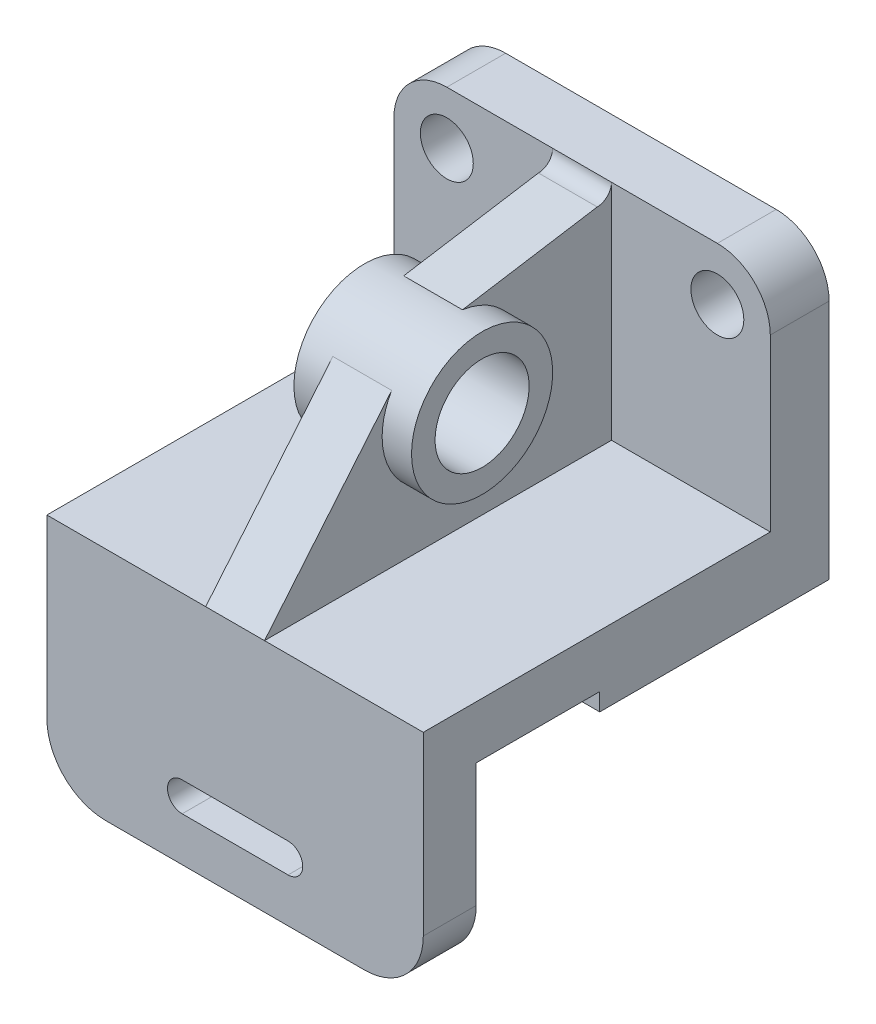
ISO-10303-21;
HEADER;
FILE_DESCRIPTION(('STEP AP214'),'2;1');
FILE_NAME('part.step','',(''),(''),'','','');
FILE_SCHEMA(('AUTOMOTIVE_DESIGN { 1 0 10303 214 1 1 1 1 }'));
ENDSEC;
DATA;
#1=APPLICATION_CONTEXT('core data for automotive mechanical design processes');
#2=APPLICATION_PROTOCOL_DEFINITION('international standard','automotive_design',2000,#1);
#3=PRODUCT_CONTEXT('',#1,'mechanical');
#4=PRODUCT('Part','Part','',(#3));
#5=PRODUCT_RELATED_PRODUCT_CATEGORY('part','',(#4));
#6=PRODUCT_DEFINITION_FORMATION('','',#4);
#7=PRODUCT_DEFINITION_CONTEXT('part definition',#1,'design');
#8=PRODUCT_DEFINITION('design','',#6,#7);
#9=PRODUCT_DEFINITION_SHAPE('','',#8);
#10=(LENGTH_UNIT() NAMED_UNIT(*) SI_UNIT(.MILLI.,.METRE.));
#11=(NAMED_UNIT(*) PLANE_ANGLE_UNIT() SI_UNIT($,.RADIAN.));
#12=(NAMED_UNIT(*) SI_UNIT($,.STERADIAN.) SOLID_ANGLE_UNIT());
#13=UNCERTAINTY_MEASURE_WITH_UNIT(LENGTH_MEASURE(1.E-05),#10,'distance_accuracy_value','');
#14=(GEOMETRIC_REPRESENTATION_CONTEXT(3) GLOBAL_UNCERTAINTY_ASSIGNED_CONTEXT((#13)) GLOBAL_UNIT_ASSIGNED_CONTEXT((#10,
#11,#12)) REPRESENTATION_CONTEXT('',''));
#15=CARTESIAN_POINT('',(0.,0.,0.));
#16=DIRECTION('',(0.,0.,1.));
#17=DIRECTION('',(1.,0.,0.));
#18=AXIS2_PLACEMENT_3D('',#15,#16,#17);
#19=CARTESIAN_POINT('',(27.,12.,69.));
#20=DIRECTION('',(0.,-0.639017565065654,-0.769192142144966));
#21=DIRECTION('',(0.,0.769192142144966,-0.639017565065655));
#22=AXIS2_PLACEMENT_3D('',#19,#20,#21);
#23=PLANE('',#22);
#24=DIRECTION('',(1.,0.,0.));
#25=VECTOR('',#24,1.);
#26=CARTESIAN_POINT('',(22.,38.0310911105716,47.3742922657878));
#27=LINE('',#26,#25);
#28=CARTESIAN_POINT('',(27.,38.0310911105716,47.3742922657878));
#29=VERTEX_POINT('',#28);
#30=CARTESIAN_POINT('',(37.,38.0310911105716,47.3742922657878));
#31=VERTEX_POINT('',#30);
#32=EDGE_CURVE('E359',#29,#31,#27,.T.);
#33=ORIENTED_EDGE('',*,*,#32,.F.);
#34=DIRECTION('',(0.,0.769192142144966,-0.639017565065654));
#35=VECTOR('',#34,1.);
#36=CARTESIAN_POINT('',(27.,12.,69.));
#37=LINE('',#36,#35);
#38=CARTESIAN_POINT('',(27.,12.,69.));
#39=VERTEX_POINT('',#38);
#40=EDGE_CURVE('E372',#39,#29,#37,.T.);
#41=ORIENTED_EDGE('',*,*,#40,.F.);
#42=DIRECTION('',(1.,0.,0.));
#43=VECTOR('',#42,1.);
#44=CARTESIAN_POINT('',(27.,12.,69.));
#45=LINE('',#44,#43);
#46=CARTESIAN_POINT('',(37.,12.,69.));
#47=VERTEX_POINT('',#46);
#48=EDGE_CURVE('E402',#39,#47,#45,.T.);
#49=ORIENTED_EDGE('',*,*,#48,.T.);
#50=DIRECTION('',(0.,0.769192142144966,-0.639017565065654));
#51=VECTOR('',#50,1.);
#52=CARTESIAN_POINT('',(37.,12.,69.));
#53=LINE('',#52,#51);
#54=EDGE_CURVE('E390',#47,#31,#53,.T.);
#55=ORIENTED_EDGE('',*,*,#54,.T.);
#56=EDGE_LOOP('',(#33,#41,#49,#55));
#57=FACE_BOUND('',#56,.T.);
#58=ADVANCED_FACE('F39',(#57),#23,.F.);
#59=CARTESIAN_POINT('',(9.,41.,10.));
#60=DIRECTION('',(0.,0.,-1.));
#61=DIRECTION('',(-1.,0.,0.));
#62=AXIS2_PLACEMENT_3D('',#59,#60,#61);
#63=PLANE('',#62);
#64=CARTESIAN_POINT('',(55.,41.,10.));
#65=DIRECTION('',(0.,0.,1.));
#66=DIRECTION('',(1.,0.,0.));
#67=AXIS2_PLACEMENT_3D('',#64,#65,#66);
#68=CIRCLE('',#67,4.5);
#69=CARTESIAN_POINT('',(59.5,41.,10.));
#70=VERTEX_POINT('',#69);
#71=EDGE_CURVE('E272',#70,#70,#68,.T.);
#72=ORIENTED_EDGE('',*,*,#71,.F.);
#73=EDGE_LOOP('',(#72));
#74=FACE_BOUND('',#73,.T.);
#75=DIRECTION('',(0.,-1.,0.));
#76=VECTOR('',#75,1.);
#77=CARTESIAN_POINT('',(37.,12.,10.));
#78=LINE('',#77,#76);
#79=CARTESIAN_POINT('',(37.,50.,10.));
#80=VERTEX_POINT('',#79);
#81=CARTESIAN_POINT('',(37.,12.,10.));
#82=VERTEX_POINT('',#81);
#83=EDGE_CURVE('E370',#80,#82,#78,.T.);
#84=ORIENTED_EDGE('',*,*,#83,.T.);
#85=DIRECTION('',(1.,0.,0.));
#86=VECTOR('',#85,1.);
#87=CARTESIAN_POINT('',(9.,12.,10.));
#88=LINE('',#87,#86);
#89=CARTESIAN_POINT('',(64.,12.,10.));
#90=VERTEX_POINT('',#89);
#91=EDGE_CURVE('E273',#82,#90,#88,.T.);
#92=ORIENTED_EDGE('',*,*,#91,.T.);
#93=DIRECTION('',(0.,1.,0.));
#94=VECTOR('',#93,1.);
#95=CARTESIAN_POINT('',(64.,41.,10.));
#96=LINE('',#95,#94);
#97=CARTESIAN_POINT('',(64.,41.,10.));
#98=VERTEX_POINT('',#97);
#99=EDGE_CURVE('E290',#90,#98,#96,.T.);
#100=ORIENTED_EDGE('',*,*,#99,.T.);
#101=CARTESIAN_POINT('',(55.,41.,10.));
#102=DIRECTION('',(0.,0.,1.));
#103=DIRECTION('',(-1.,0.,0.));
#104=AXIS2_PLACEMENT_3D('',#101,#102,#103);
#105=CIRCLE('',#104,9.00000000000001);
#106=CARTESIAN_POINT('',(55.,50.,10.));
#107=VERTEX_POINT('',#106);
#108=EDGE_CURVE('E287',#98,#107,#105,.T.);
#109=ORIENTED_EDGE('',*,*,#108,.T.);
#110=DIRECTION('',(-1.,0.,0.));
#111=VECTOR('',#110,1.);
#112=CARTESIAN_POINT('',(9.,50.,10.));
#113=LINE('',#112,#111);
#114=EDGE_CURVE('E291',#107,#80,#113,.T.);
#115=ORIENTED_EDGE('',*,*,#114,.T.);
#116=EDGE_LOOP('',(#84,#92,#100,#109,#115));
#117=FACE_BOUND('',#116,.T.);
#118=ADVANCED_FACE('F477',(#74,#117),#63,.F.);
#119=CARTESIAN_POINT('',(64.,12.,0.));
#120=DIRECTION('',(0.,1.,0.));
#121=DIRECTION('',(0.,0.,1.));
#122=AXIS2_PLACEMENT_3D('',#119,#120,#121);
#123=PLANE('',#122);
#124=ORIENTED_EDGE('',*,*,#91,.F.);
#125=DIRECTION('',(0.,0.,1.));
#126=VECTOR('',#125,1.);
#127=CARTESIAN_POINT('',(37.,12.,10.));
#128=LINE('',#127,#126);
#129=EDGE_CURVE('E383',#82,#47,#128,.T.);
#130=ORIENTED_EDGE('',*,*,#129,.T.);
#131=DIRECTION('',(-1.,0.,0.));
#132=VECTOR('',#131,1.);
#133=CARTESIAN_POINT('',(64.,12.,69.));
#134=LINE('',#133,#132);
#135=CARTESIAN_POINT('',(64.,12.,69.));
#136=VERTEX_POINT('',#135);
#137=EDGE_CURVE('E260',#136,#47,#134,.T.);
#138=ORIENTED_EDGE('',*,*,#137,.F.);
#139=DIRECTION('',(0.,0.,-1.));
#140=VECTOR('',#139,1.);
#141=CARTESIAN_POINT('',(64.,12.,0.));
#142=LINE('',#141,#140);
#143=EDGE_CURVE('E267',#136,#90,#142,.T.);
#144=ORIENTED_EDGE('',*,*,#143,.T.);
#145=EDGE_LOOP('',(#124,#130,#138,#144));
#146=FACE_BOUND('',#145,.T.);
#147=ADVANCED_FACE('F490',(#146),#123,.T.);
#148=CARTESIAN_POINT('',(64.,0.,10.));
#149=DIRECTION('',(0.,1.,0.));
#150=DIRECTION('',(-1.,0.,0.));
#151=AXIS2_PLACEMENT_3D('',#148,#149,#150);
#152=PLANE('',#151);
#153=DIRECTION('',(1.,0.,0.));
#154=VECTOR('',#153,1.);
#155=CARTESIAN_POINT('',(64.,0.,0.));
#156=LINE('',#155,#154);
#157=CARTESIAN_POINT('',(0.,0.,0.));
#158=VERTEX_POINT('',#157);
#159=CARTESIAN_POINT('',(64.,0.,0.));
#160=VERTEX_POINT('',#159);
#161=EDGE_CURVE('E279',#158,#160,#156,.T.);
#162=ORIENTED_EDGE('',*,*,#161,.T.);
#163=DIRECTION('',(0.,0.,-1.));
#164=VECTOR('',#163,1.);
#165=CARTESIAN_POINT('',(64.,0.,10.));
#166=LINE('',#165,#164);
#167=CARTESIAN_POINT('',(64.,0.,39.));
#168=VERTEX_POINT('',#167);
#169=EDGE_CURVE('E326',#168,#160,#166,.T.);
#170=ORIENTED_EDGE('',*,*,#169,.F.);
#171=DIRECTION('',(-1.,0.,0.));
#172=VECTOR('',#171,1.);
#173=CARTESIAN_POINT('',(64.,0.,39.));
#174=LINE('',#173,#172);
#175=CARTESIAN_POINT('',(0.,0.,39.));
#176=VERTEX_POINT('',#175);
#177=EDGE_CURVE('E266',#168,#176,#174,.T.);
#178=ORIENTED_EDGE('',*,*,#177,.T.);
#179=DIRECTION('',(0.,0.,-1.));
#180=VECTOR('',#179,1.);
#181=CARTESIAN_POINT('',(0.,0.,10.));
#182=LINE('',#181,#180);
#183=EDGE_CURVE('E297',#176,#158,#182,.T.);
#184=ORIENTED_EDGE('',*,*,#183,.T.);
#185=EDGE_LOOP('',(#162,#170,#178,#184));
#186=FACE_BOUND('',#185,.T.);
#187=ADVANCED_FACE('F454',(#186),#152,.F.);
#188=CARTESIAN_POINT('',(64.,41.,10.));
#189=DIRECTION('',(-1.,0.,0.));
#190=DIRECTION('',(0.,-1.,0.));
#191=AXIS2_PLACEMENT_3D('',#188,#189,#190);
#192=PLANE('',#191);
#193=DIRECTION('',(0.,1.,0.));
#194=VECTOR('',#193,1.);
#195=CARTESIAN_POINT('',(64.,12.,69.));
#196=LINE('',#195,#194);
#197=CARTESIAN_POINT('',(64.,-18.,69.));
#198=VERTEX_POINT('',#197);
#199=EDGE_CURVE('E413',#198,#136,#196,.T.);
#200=ORIENTED_EDGE('',*,*,#199,.F.);
#201=DIRECTION('',(0.,0.,1.));
#202=VECTOR('',#201,1.);
#203=CARTESIAN_POINT('',(64.,-18.,60.));
#204=LINE('',#203,#202);
#205=CARTESIAN_POINT('',(64.,-18.,60.));
#206=VERTEX_POINT('',#205);
#207=EDGE_CURVE('E50',#198,#206,#204,.F.);
#208=ORIENTED_EDGE('',*,*,#207,.T.);
#209=DIRECTION('',(0.,-1.,0.));
#210=VECTOR('',#209,1.);
#211=CARTESIAN_POINT('',(64.,3.,60.));
#212=LINE('',#211,#210);
#213=CARTESIAN_POINT('',(64.,3.,60.));
#214=VERTEX_POINT('',#213);
#215=EDGE_CURVE('E411',#214,#206,#212,.T.);
#216=ORIENTED_EDGE('',*,*,#215,.F.);
#217=DIRECTION('',(0.,0.,1.));
#218=VECTOR('',#217,1.);
#219=CARTESIAN_POINT('',(64.,3.,39.));
#220=LINE('',#219,#218);
#221=CARTESIAN_POINT('',(64.,3.,39.));
#222=VERTEX_POINT('',#221);
#223=EDGE_CURVE('E410',#222,#214,#220,.T.);
#224=ORIENTED_EDGE('',*,*,#223,.F.);
#225=DIRECTION('',(0.,1.,0.));
#226=VECTOR('',#225,1.);
#227=CARTESIAN_POINT('',(64.,0.,39.));
#228=LINE('',#227,#226);
#229=EDGE_CURVE('E404',#168,#222,#228,.T.);
#230=ORIENTED_EDGE('',*,*,#229,.F.);
#231=ORIENTED_EDGE('',*,*,#169,.T.);
#232=DIRECTION('',(0.,1.,0.));
#233=VECTOR('',#232,1.);
#234=CARTESIAN_POINT('',(64.,41.,0.));
#235=LINE('',#234,#233);
#236=CARTESIAN_POINT('',(64.,41.,0.));
#237=VERTEX_POINT('',#236);
#238=EDGE_CURVE('E303',#160,#237,#235,.T.);
#239=ORIENTED_EDGE('',*,*,#238,.T.);
#240=DIRECTION('',(0.,0.,-1.));
#241=VECTOR('',#240,1.);
#242=CARTESIAN_POINT('',(64.,41.,10.));
#243=LINE('',#242,#241);
#244=EDGE_CURVE('E323',#98,#237,#243,.T.);
#245=ORIENTED_EDGE('',*,*,#244,.F.);
#246=ORIENTED_EDGE('',*,*,#99,.F.);
#247=ORIENTED_EDGE('',*,*,#143,.F.);
#248=EDGE_LOOP('',(#200,#208,#216,#224,#230,#231,#239,#245,#246,#247));
#249=FACE_BOUND('',#248,.T.);
#250=ADVANCED_FACE('F526',(#249),#192,.F.);
#251=CARTESIAN_POINT('',(55.,41.,10.));
#252=DIRECTION('',(0.,0.,-1.));
#253=DIRECTION('',(-1.,0.,0.));
#254=AXIS2_PLACEMENT_3D('',#251,#252,#253);
#255=CYLINDRICAL_SURFACE('',#254,9.00000000000001);
#256=CARTESIAN_POINT('',(55.,41.,0.));
#257=DIRECTION('',(0.,0.,1.));
#258=DIRECTION('',(-1.,0.,0.));
#259=AXIS2_PLACEMENT_3D('',#256,#257,#258);
#260=CIRCLE('',#259,9.00000000000001);
#261=CARTESIAN_POINT('',(55.,50.,0.));
#262=VERTEX_POINT('',#261);
#263=EDGE_CURVE('E304',#237,#262,#260,.T.);
#264=ORIENTED_EDGE('',*,*,#263,.T.);
#265=DIRECTION('',(0.,0.,-1.));
#266=VECTOR('',#265,1.);
#267=CARTESIAN_POINT('',(55.,50.,10.));
#268=LINE('',#267,#266);
#269=EDGE_CURVE('E319',#107,#262,#268,.T.);
#270=ORIENTED_EDGE('',*,*,#269,.F.);
#271=ORIENTED_EDGE('',*,*,#108,.F.);
#272=ORIENTED_EDGE('',*,*,#244,.T.);
#273=EDGE_LOOP('',(#264,#270,#271,#272));
#274=FACE_BOUND('',#273,.T.);
#275=ADVANCED_FACE('F522',(#274),#255,.T.);
#276=CARTESIAN_POINT('',(9.,50.,10.));
#277=DIRECTION('',(0.,-1.,0.));
#278=DIRECTION('',(1.,0.,0.));
#279=AXIS2_PLACEMENT_3D('',#276,#277,#278);
#280=PLANE('',#279);
#281=DIRECTION('',(-1.,0.,0.));
#282=VECTOR('',#281,1.);
#283=CARTESIAN_POINT('',(9.,50.,0.));
#284=LINE('',#283,#282);
#285=CARTESIAN_POINT('',(9.,50.,0.));
#286=VERTEX_POINT('',#285);
#287=EDGE_CURVE('E307',#262,#286,#284,.T.);
#288=ORIENTED_EDGE('',*,*,#287,.T.);
#289=DIRECTION('',(0.,0.,-1.));
#290=VECTOR('',#289,1.);
#291=CARTESIAN_POINT('',(9.,50.,10.));
#292=LINE('',#291,#290);
#293=CARTESIAN_POINT('',(9.,50.,10.));
#294=VERTEX_POINT('',#293);
#295=EDGE_CURVE('E320',#294,#286,#292,.T.);
#296=ORIENTED_EDGE('',*,*,#295,.F.);
#297=CARTESIAN_POINT('',(27.,50.,10.));
#298=VERTEX_POINT('',#297);
#299=EDGE_CURVE('E295',#298,#294,#113,.T.);
#300=ORIENTED_EDGE('',*,*,#299,.F.);
#301=DIRECTION('',(1.,0.,0.));
#302=VECTOR('',#301,1.);
#303=CARTESIAN_POINT('',(27.,50.,10.));
#304=LINE('',#303,#302);
#305=EDGE_CURVE('E381',#298,#80,#304,.T.);
#306=ORIENTED_EDGE('',*,*,#305,.T.);
#307=ORIENTED_EDGE('',*,*,#114,.F.);
#308=ORIENTED_EDGE('',*,*,#269,.T.);
#309=EDGE_LOOP('',(#288,#296,#300,#306,#307,#308));
#310=FACE_BOUND('',#309,.T.);
#311=ADVANCED_FACE('F521',(#310),#280,.F.);
#312=CARTESIAN_POINT('',(9.,41.,10.));
#313=DIRECTION('',(0.,0.,-1.));
#314=DIRECTION('',(-1.,0.,0.));
#315=AXIS2_PLACEMENT_3D('',#312,#313,#314);
#316=CYLINDRICAL_SURFACE('',#315,9.);
#317=CARTESIAN_POINT('',(9.,41.,0.));
#318=DIRECTION('',(0.,0.,1.));
#319=DIRECTION('',(-1.,0.,0.));
#320=AXIS2_PLACEMENT_3D('',#317,#318,#319);
#321=CIRCLE('',#320,9.);
#322=CARTESIAN_POINT('',(0.,41.,0.));
#323=VERTEX_POINT('',#322);
#324=EDGE_CURVE('E310',#286,#323,#321,.T.);
#325=ORIENTED_EDGE('',*,*,#324,.T.);
#326=DIRECTION('',(0.,0.,-1.));
#327=VECTOR('',#326,1.);
#328=CARTESIAN_POINT('',(0.,41.,10.));
#329=LINE('',#328,#327);
#330=CARTESIAN_POINT('',(0.,41.,10.));
#331=VERTEX_POINT('',#330);
#332=EDGE_CURVE('E314',#331,#323,#329,.T.);
#333=ORIENTED_EDGE('',*,*,#332,.F.);
#334=CARTESIAN_POINT('',(9.,41.,10.));
#335=DIRECTION('',(0.,0.,1.));
#336=DIRECTION('',(-1.,0.,0.));
#337=AXIS2_PLACEMENT_3D('',#334,#335,#336);
#338=CIRCLE('',#337,9.);
#339=EDGE_CURVE('E298',#294,#331,#338,.T.);
#340=ORIENTED_EDGE('',*,*,#339,.F.);
#341=ORIENTED_EDGE('',*,*,#295,.T.);
#342=EDGE_LOOP('',(#325,#333,#340,#341));
#343=FACE_BOUND('',#342,.T.);
#344=ADVANCED_FACE('F443',(#343),#316,.T.);
#345=CARTESIAN_POINT('',(0.,0.,10.));
#346=DIRECTION('',(1.,0.,0.));
#347=DIRECTION('',(0.,0.,-1.));
#348=AXIS2_PLACEMENT_3D('',#345,#346,#347);
#349=PLANE('',#348);
#350=DIRECTION('',(0.,-1.,0.));
#351=VECTOR('',#350,1.);
#352=CARTESIAN_POINT('',(0.,3.,60.));
#353=LINE('',#352,#351);
#354=CARTESIAN_POINT('',(0.,3.,60.));
#355=VERTEX_POINT('',#354);
#356=CARTESIAN_POINT('',(0.,-18.,60.));
#357=VERTEX_POINT('',#356);
#358=EDGE_CURVE('E425',#355,#357,#353,.T.);
#359=ORIENTED_EDGE('',*,*,#358,.T.);
#360=DIRECTION('',(0.,0.,1.));
#361=VECTOR('',#360,1.);
#362=CARTESIAN_POINT('',(0.,-18.,69.));
#363=LINE('',#362,#361);
#364=CARTESIAN_POINT('',(0.,-18.,69.));
#365=VERTEX_POINT('',#364);
#366=EDGE_CURVE('E223',#357,#365,#363,.T.);
#367=ORIENTED_EDGE('',*,*,#366,.T.);
#368=DIRECTION('',(0.,1.,0.));
#369=VECTOR('',#368,1.);
#370=CARTESIAN_POINT('',(0.,12.,69.));
#371=LINE('',#370,#369);
#372=CARTESIAN_POINT('',(0.,12.,69.));
#373=VERTEX_POINT('',#372);
#374=EDGE_CURVE('E422',#365,#373,#371,.T.);
#375=ORIENTED_EDGE('',*,*,#374,.T.);
#376=DIRECTION('',(0.,0.,-1.));
#377=VECTOR('',#376,1.);
#378=CARTESIAN_POINT('',(0.,12.,0.));
#379=LINE('',#378,#377);
#380=CARTESIAN_POINT('',(0.,12.,10.));
#381=VERTEX_POINT('',#380);
#382=EDGE_CURVE('E406',#373,#381,#379,.T.);
#383=ORIENTED_EDGE('',*,*,#382,.T.);
#384=DIRECTION('',(0.,-1.,0.));
#385=VECTOR('',#384,1.);
#386=CARTESIAN_POINT('',(0.,0.,10.));
#387=LINE('',#386,#385);
#388=EDGE_CURVE('E296',#331,#381,#387,.T.);
#389=ORIENTED_EDGE('',*,*,#388,.F.);
#390=ORIENTED_EDGE('',*,*,#332,.T.);
#391=DIRECTION('',(0.,-1.,0.));
#392=VECTOR('',#391,1.);
#393=CARTESIAN_POINT('',(0.,0.,0.));
#394=LINE('',#393,#392);
#395=EDGE_CURVE('E289',#323,#158,#394,.T.);
#396=ORIENTED_EDGE('',*,*,#395,.T.);
#397=ORIENTED_EDGE('',*,*,#183,.F.);
#398=DIRECTION('',(0.,1.,0.));
#399=VECTOR('',#398,1.);
#400=CARTESIAN_POINT('',(0.,0.,39.));
#401=LINE('',#400,#399);
#402=CARTESIAN_POINT('',(0.,3.,39.));
#403=VERTEX_POINT('',#402);
#404=EDGE_CURVE('E401',#176,#403,#401,.T.);
#405=ORIENTED_EDGE('',*,*,#404,.T.);
#406=DIRECTION('',(0.,0.,1.));
#407=VECTOR('',#406,1.);
#408=CARTESIAN_POINT('',(0.,3.,39.));
#409=LINE('',#408,#407);
#410=EDGE_CURVE('E420',#403,#355,#409,.T.);
#411=ORIENTED_EDGE('',*,*,#410,.T.);
#412=EDGE_LOOP('',(#359,#367,#375,#383,#389,#390,#396,#397,#405,#411));
#413=FACE_BOUND('',#412,.T.);
#414=ADVANCED_FACE('F429',(#413),#349,.F.);
#415=CARTESIAN_POINT('',(9.,41.,10.));
#416=DIRECTION('',(0.,0.,1.));
#417=DIRECTION('',(1.,0.,0.));
#418=AXIS2_PLACEMENT_3D('',#415,#416,#417);
#419=CIRCLE('',#418,4.5);
#420=CARTESIAN_POINT('',(13.5,41.,10.));
#421=VERTEX_POINT('',#420);
#422=EDGE_CURVE('E276',#421,#421,#419,.T.);
#423=ORIENTED_EDGE('',*,*,#422,.F.);
#424=EDGE_LOOP('',(#423));
#425=FACE_BOUND('',#424,.T.);
#426=CARTESIAN_POINT('',(27.,12.,10.));
#427=VERTEX_POINT('',#426);
#428=EDGE_CURVE('E269',#381,#427,#88,.T.);
#429=ORIENTED_EDGE('',*,*,#428,.T.);
#430=DIRECTION('',(0.,-1.,0.));
#431=VECTOR('',#430,1.);
#432=CARTESIAN_POINT('',(27.,12.,10.));
#433=LINE('',#432,#431);
#434=EDGE_CURVE('E366',#298,#427,#433,.T.);
#435=ORIENTED_EDGE('',*,*,#434,.F.);
#436=ORIENTED_EDGE('',*,*,#299,.T.);
#437=ORIENTED_EDGE('',*,*,#339,.T.);
#438=ORIENTED_EDGE('',*,*,#388,.T.);
#439=EDGE_LOOP('',(#429,#435,#436,#437,#438));
#440=FACE_BOUND('',#439,.T.);
#441=ADVANCED_FACE('F438',(#425,#440),#63,.F.);
#442=CARTESIAN_POINT('',(9.,41.,0.));
#443=DIRECTION('',(0.,0.,-1.));
#444=DIRECTION('',(-1.,0.,0.));
#445=AXIS2_PLACEMENT_3D('',#442,#443,#444);
#446=PLANE('',#445);
#447=ORIENTED_EDGE('',*,*,#263,.F.);
#448=ORIENTED_EDGE('',*,*,#238,.F.);
#449=ORIENTED_EDGE('',*,*,#161,.F.);
#450=ORIENTED_EDGE('',*,*,#395,.F.);
#451=ORIENTED_EDGE('',*,*,#324,.F.);
#452=ORIENTED_EDGE('',*,*,#287,.F.);
#453=EDGE_LOOP('',(#447,#448,#449,#450,#451,#452));
#454=FACE_BOUND('',#453,.T.);
#455=CARTESIAN_POINT('',(9.,41.,0.));
#456=DIRECTION('',(0.,0.,1.));
#457=DIRECTION('',(1.,0.,0.));
#458=AXIS2_PLACEMENT_3D('',#455,#456,#457);
#459=CIRCLE('',#458,4.5);
#460=CARTESIAN_POINT('',(13.5,41.,0.));
#461=VERTEX_POINT('',#460);
#462=EDGE_CURVE('E274',#461,#461,#459,.T.);
#463=ORIENTED_EDGE('',*,*,#462,.T.);
#464=EDGE_LOOP('',(#463));
#465=FACE_BOUND('',#464,.T.);
#466=CARTESIAN_POINT('',(55.,41.,0.));
#467=DIRECTION('',(0.,0.,1.));
#468=DIRECTION('',(1.,0.,0.));
#469=AXIS2_PLACEMENT_3D('',#466,#467,#468);
#470=CIRCLE('',#469,4.5);
#471=CARTESIAN_POINT('',(59.5,41.,0.));
#472=VERTEX_POINT('',#471);
#473=EDGE_CURVE('E285',#472,#472,#470,.T.);
#474=ORIENTED_EDGE('',*,*,#473,.T.);
#475=EDGE_LOOP('',(#474));
#476=FACE_BOUND('',#475,.T.);
#477=ADVANCED_FACE('F451',(#454,#465,#476),#446,.T.);
#478=CARTESIAN_POINT('',(55.,41.,0.));
#479=DIRECTION('',(0.,0.,1.));
#480=DIRECTION('',(1.,0.,0.));
#481=AXIS2_PLACEMENT_3D('',#478,#479,#480);
#482=CYLINDRICAL_SURFACE('',#481,4.5);
#483=ORIENTED_EDGE('',*,*,#473,.F.);
#484=EDGE_LOOP('',(#483));
#485=FACE_BOUND('',#484,.T.);
#486=ORIENTED_EDGE('',*,*,#71,.T.);
#487=EDGE_LOOP('',(#486));
#488=FACE_BOUND('',#487,.T.);
#489=ADVANCED_FACE('F507',(#485,#488),#482,.F.);
#490=CARTESIAN_POINT('',(9.,41.,0.));
#491=DIRECTION('',(0.,0.,1.));
#492=DIRECTION('',(1.,0.,0.));
#493=AXIS2_PLACEMENT_3D('',#490,#491,#492);
#494=CYLINDRICAL_SURFACE('',#493,4.5);
#495=ORIENTED_EDGE('',*,*,#462,.F.);
#496=EDGE_LOOP('',(#495));
#497=FACE_BOUND('',#496,.T.);
#498=ORIENTED_EDGE('',*,*,#422,.T.);
#499=EDGE_LOOP('',(#498));
#500=FACE_BOUND('',#499,.T.);
#501=ADVANCED_FACE('F497',(#497,#500),#494,.F.);
#502=DIRECTION('',(0.,0.,1.));
#503=VECTOR('',#502,1.);
#504=CARTESIAN_POINT('',(27.,12.,10.));
#505=LINE('',#504,#503);
#506=EDGE_CURVE('E367',#427,#39,#505,.T.);
#507=ORIENTED_EDGE('',*,*,#506,.F.);
#508=ORIENTED_EDGE('',*,*,#428,.F.);
#509=ORIENTED_EDGE('',*,*,#382,.F.);
#510=EDGE_CURVE('E255',#39,#373,#134,.T.);
#511=ORIENTED_EDGE('',*,*,#510,.F.);
#512=EDGE_LOOP('',(#507,#508,#509,#511));
#513=FACE_BOUND('',#512,.T.);
#514=ADVANCED_FACE('F434',(#513),#123,.T.);
#515=CARTESIAN_POINT('',(64.,12.,69.));
#516=DIRECTION('',(0.,0.,1.));
#517=DIRECTION('',(0.,-1.,0.));
#518=AXIS2_PLACEMENT_3D('',#515,#516,#517);
#519=PLANE('',#518);
#520=CARTESIAN_POINT('',(23.,-18.,69.));
#521=DIRECTION('',(0.,0.,1.));
#522=DIRECTION('',(0.,-1.,0.));
#523=AXIS2_PLACEMENT_3D('',#520,#521,#522);
#524=CIRCLE('',#523,2.5);
#525=CARTESIAN_POINT('',(23.,-15.5,69.));
#526=VERTEX_POINT('',#525);
#527=CARTESIAN_POINT('',(23.,-20.5,69.));
#528=VERTEX_POINT('',#527);
#529=EDGE_CURVE('E217',#526,#528,#524,.T.);
#530=ORIENTED_EDGE('',*,*,#529,.F.);
#531=DIRECTION('',(-1.,0.,0.));
#532=VECTOR('',#531,1.);
#533=CARTESIAN_POINT('',(64.,-15.5,69.));
#534=LINE('',#533,#532);
#535=CARTESIAN_POINT('',(41.,-15.5,69.));
#536=VERTEX_POINT('',#535);
#537=EDGE_CURVE('E353',#536,#526,#534,.T.);
#538=ORIENTED_EDGE('',*,*,#537,.F.);
#539=CARTESIAN_POINT('',(41.,-18.,69.));
#540=DIRECTION('',(0.,0.,1.));
#541=DIRECTION('',(0.,-1.,0.));
#542=AXIS2_PLACEMENT_3D('',#539,#540,#541);
#543=CIRCLE('',#542,2.5);
#544=CARTESIAN_POINT('',(41.,-20.5,69.));
#545=VERTEX_POINT('',#544);
#546=EDGE_CURVE('E337',#545,#536,#543,.T.);
#547=ORIENTED_EDGE('',*,*,#546,.F.);
#548=DIRECTION('',(1.,0.,0.));
#549=VECTOR('',#548,1.);
#550=CARTESIAN_POINT('',(64.,-20.5,69.));
#551=LINE('',#550,#549);
#552=EDGE_CURVE('E344',#528,#545,#551,.T.);
#553=ORIENTED_EDGE('',*,*,#552,.F.);
#554=EDGE_LOOP('',(#530,#538,#547,#553));
#555=FACE_BOUND('',#554,.T.);
#556=DIRECTION('',(-1.,0.,0.));
#557=VECTOR('',#556,1.);
#558=CARTESIAN_POINT('',(64.,-28.,69.));
#559=LINE('',#558,#557);
#560=CARTESIAN_POINT('',(54.,-28.,69.));
#561=VERTEX_POINT('',#560);
#562=CARTESIAN_POINT('',(10.,-28.,69.));
#563=VERTEX_POINT('',#562);
#564=EDGE_CURVE('E250',#561,#563,#559,.T.);
#565=ORIENTED_EDGE('',*,*,#564,.F.);
#566=CARTESIAN_POINT('',(54.,-18.,69.));
#567=DIRECTION('',(0.,0.,1.));
#568=DIRECTION('',(0.,-1.,0.));
#569=AXIS2_PLACEMENT_3D('',#566,#567,#568);
#570=CIRCLE('',#569,10.);
#571=EDGE_CURVE('E63',#561,#198,#570,.T.);
#572=ORIENTED_EDGE('',*,*,#571,.T.);
#573=ORIENTED_EDGE('',*,*,#199,.T.);
#574=ORIENTED_EDGE('',*,*,#137,.T.);
#575=ORIENTED_EDGE('',*,*,#48,.F.);
#576=ORIENTED_EDGE('',*,*,#510,.T.);
#577=ORIENTED_EDGE('',*,*,#374,.F.);
#578=CARTESIAN_POINT('',(10.,-18.,69.));
#579=DIRECTION('',(0.,0.,1.));
#580=DIRECTION('',(0.,-1.,0.));
#581=AXIS2_PLACEMENT_3D('',#578,#579,#580);
#582=CIRCLE('',#581,10.);
#583=EDGE_CURVE('E226',#365,#563,#582,.T.);
#584=ORIENTED_EDGE('',*,*,#583,.T.);
#585=EDGE_LOOP('',(#565,#572,#573,#574,#575,#576,#577,#584));
#586=FACE_BOUND('',#585,.T.);
#587=ADVANCED_FACE('F253',(#555,#586),#519,.T.);
#588=CARTESIAN_POINT('',(64.,-28.,60.));
#589=DIRECTION('',(0.,-1.,0.));
#590=DIRECTION('',(0.,0.,-1.));
#591=AXIS2_PLACEMENT_3D('',#588,#589,#590);
#592=PLANE('',#591);
#593=DIRECTION('',(-1.,0.,0.));
#594=VECTOR('',#593,1.);
#595=CARTESIAN_POINT('',(64.,-28.,60.));
#596=LINE('',#595,#594);
#597=CARTESIAN_POINT('',(54.,-28.,60.));
#598=VERTEX_POINT('',#597);
#599=CARTESIAN_POINT('',(10.,-28.,60.));
#600=VERTEX_POINT('',#599);
#601=EDGE_CURVE('E248',#598,#600,#596,.T.);
#602=ORIENTED_EDGE('',*,*,#601,.F.);
#603=DIRECTION('',(0.,0.,1.));
#604=VECTOR('',#603,1.);
#605=CARTESIAN_POINT('',(54.,-28.,69.));
#606=LINE('',#605,#604);
#607=EDGE_CURVE('E238',#598,#561,#606,.T.);
#608=ORIENTED_EDGE('',*,*,#607,.T.);
#609=ORIENTED_EDGE('',*,*,#564,.T.);
#610=DIRECTION('',(0.,0.,1.));
#611=VECTOR('',#610,1.);
#612=CARTESIAN_POINT('',(10.,-28.,60.));
#613=LINE('',#612,#611);
#614=EDGE_CURVE('E234',#563,#600,#613,.F.);
#615=ORIENTED_EDGE('',*,*,#614,.T.);
#616=EDGE_LOOP('',(#602,#608,#609,#615));
#617=FACE_BOUND('',#616,.T.);
#618=ADVANCED_FACE('F246',(#617),#592,.T.);
#619=CARTESIAN_POINT('',(64.,3.,60.));
#620=DIRECTION('',(0.,0.,-1.));
#621=DIRECTION('',(-1.,0.,0.));
#622=AXIS2_PLACEMENT_3D('',#619,#620,#621);
#623=PLANE('',#622);
#624=CARTESIAN_POINT('',(23.,-18.,60.));
#625=DIRECTION('',(0.,0.,-1.));
#626=DIRECTION('',(-1.,0.,0.));
#627=AXIS2_PLACEMENT_3D('',#624,#625,#626);
#628=CIRCLE('',#627,2.5);
#629=CARTESIAN_POINT('',(23.,-20.5,60.));
#630=VERTEX_POINT('',#629);
#631=CARTESIAN_POINT('',(23.,-15.5,60.));
#632=VERTEX_POINT('',#631);
#633=EDGE_CURVE('E214',#630,#632,#628,.T.);
#634=ORIENTED_EDGE('',*,*,#633,.F.);
#635=DIRECTION('',(-1.,0.,0.));
#636=VECTOR('',#635,1.);
#637=CARTESIAN_POINT('',(64.,-20.5,60.));
#638=LINE('',#637,#636);
#639=CARTESIAN_POINT('',(41.,-20.5,60.));
#640=VERTEX_POINT('',#639);
#641=EDGE_CURVE('E196',#640,#630,#638,.T.);
#642=ORIENTED_EDGE('',*,*,#641,.F.);
#643=CARTESIAN_POINT('',(41.,-18.,60.));
#644=DIRECTION('',(0.,0.,-1.));
#645=DIRECTION('',(-1.,0.,0.));
#646=AXIS2_PLACEMENT_3D('',#643,#644,#645);
#647=CIRCLE('',#646,2.5);
#648=CARTESIAN_POINT('',(41.,-15.5,60.));
#649=VERTEX_POINT('',#648);
#650=EDGE_CURVE('E207',#649,#640,#647,.T.);
#651=ORIENTED_EDGE('',*,*,#650,.F.);
#652=DIRECTION('',(1.,0.,0.));
#653=VECTOR('',#652,1.);
#654=CARTESIAN_POINT('',(64.,-15.5,60.));
#655=LINE('',#654,#653);
#656=EDGE_CURVE('E221',#632,#649,#655,.T.);
#657=ORIENTED_EDGE('',*,*,#656,.F.);
#658=EDGE_LOOP('',(#634,#642,#651,#657));
#659=FACE_BOUND('',#658,.T.);
#660=ORIENTED_EDGE('',*,*,#215,.T.);
#661=CARTESIAN_POINT('',(54.,-18.,60.));
#662=DIRECTION('',(0.,0.,-1.));
#663=DIRECTION('',(-1.,0.,0.));
#664=AXIS2_PLACEMENT_3D('',#661,#662,#663);
#665=CIRCLE('',#664,10.);
#666=EDGE_CURVE('E11',#206,#598,#665,.T.);
#667=ORIENTED_EDGE('',*,*,#666,.T.);
#668=ORIENTED_EDGE('',*,*,#601,.T.);
#669=CARTESIAN_POINT('',(10.,-18.,60.));
#670=DIRECTION('',(0.,0.,-1.));
#671=DIRECTION('',(-1.,0.,0.));
#672=AXIS2_PLACEMENT_3D('',#669,#670,#671);
#673=CIRCLE('',#672,10.);
#674=EDGE_CURVE('E236',#600,#357,#673,.T.);
#675=ORIENTED_EDGE('',*,*,#674,.T.);
#676=ORIENTED_EDGE('',*,*,#358,.F.);
#677=DIRECTION('',(-1.,0.,0.));
#678=VECTOR('',#677,1.);
#679=CARTESIAN_POINT('',(64.,3.,60.));
#680=LINE('',#679,#678);
#681=EDGE_CURVE('E259',#214,#355,#680,.T.);
#682=ORIENTED_EDGE('',*,*,#681,.F.);
#683=EDGE_LOOP('',(#660,#667,#668,#675,#676,#682));
#684=FACE_BOUND('',#683,.T.);
#685=ADVANCED_FACE('F225',(#659,#684),#623,.T.);
#686=CARTESIAN_POINT('',(64.,3.,39.));
#687=DIRECTION('',(0.,-1.,0.));
#688=DIRECTION('',(0.,0.,-1.));
#689=AXIS2_PLACEMENT_3D('',#686,#687,#688);
#690=PLANE('',#689);
#691=ORIENTED_EDGE('',*,*,#410,.F.);
#692=DIRECTION('',(-1.,0.,0.));
#693=VECTOR('',#692,1.);
#694=CARTESIAN_POINT('',(64.,3.,39.));
#695=LINE('',#694,#693);
#696=EDGE_CURVE('E262',#222,#403,#695,.T.);
#697=ORIENTED_EDGE('',*,*,#696,.F.);
#698=ORIENTED_EDGE('',*,*,#223,.T.);
#699=ORIENTED_EDGE('',*,*,#681,.T.);
#700=EDGE_LOOP('',(#691,#697,#698,#699));
#701=FACE_BOUND('',#700,.T.);
#702=ADVANCED_FACE('F464',(#701),#690,.T.);
#703=CARTESIAN_POINT('',(64.,0.,39.));
#704=DIRECTION('',(0.,0.,1.));
#705=DIRECTION('',(1.,0.,0.));
#706=AXIS2_PLACEMENT_3D('',#703,#704,#705);
#707=PLANE('',#706);
#708=ORIENTED_EDGE('',*,*,#404,.F.);
#709=ORIENTED_EDGE('',*,*,#177,.F.);
#710=ORIENTED_EDGE('',*,*,#229,.T.);
#711=ORIENTED_EDGE('',*,*,#696,.T.);
#712=EDGE_LOOP('',(#708,#709,#710,#711));
#713=FACE_BOUND('',#712,.T.);
#714=ADVANCED_FACE('F458',(#713),#707,.T.);
#715=CARTESIAN_POINT('',(27.,47.573393727386,12.426606272614));
#716=DIRECTION('',(0.,-0.987287345263969,-0.15894558151023));
#717=DIRECTION('',(0.,0.15894558151023,-0.987287345263969));
#718=AXIS2_PLACEMENT_3D('',#715,#716,#717);
#719=PLANE('',#718);
#720=DIRECTION('',(0.,0.15894558151023,-0.987287345263968));
#721=VECTOR('',#720,1.);
#722=CARTESIAN_POINT('',(37.,47.573393727386,12.426606272614));
#723=LINE('',#722,#721);
#724=CARTESIAN_POINT('',(37.,43.8845761722406,35.3396237757031));
#725=VERTEX_POINT('',#724);
#726=CARTESIAN_POINT('',(37.,47.573393727386,12.426606272614));
#727=VERTEX_POINT('',#726);
#728=EDGE_CURVE('E388',#725,#727,#723,.T.);
#729=ORIENTED_EDGE('',*,*,#728,.T.);
#730=DIRECTION('',(1.,0.,0.));
#731=VECTOR('',#730,1.);
#732=CARTESIAN_POINT('',(27.,47.573393727386,12.426606272614));
#733=LINE('',#732,#731);
#734=CARTESIAN_POINT('',(27.,47.573393727386,12.426606272614));
#735=VERTEX_POINT('',#734);
#736=EDGE_CURVE('E392',#735,#727,#733,.T.);
#737=ORIENTED_EDGE('',*,*,#736,.F.);
#738=DIRECTION('',(0.,0.15894558151023,-0.987287345263968));
#739=VECTOR('',#738,1.);
#740=CARTESIAN_POINT('',(27.,47.573393727386,12.426606272614));
#741=LINE('',#740,#739);
#742=CARTESIAN_POINT('',(27.,43.8845761722406,35.3396237757031));
#743=VERTEX_POINT('',#742);
#744=EDGE_CURVE('E380',#743,#735,#741,.T.);
#745=ORIENTED_EDGE('',*,*,#744,.F.);
#746=DIRECTION('',(1.,0.,0.));
#747=VECTOR('',#746,1.);
#748=CARTESIAN_POINT('',(27.,43.8845761722406,35.3396237757031));
#749=LINE('',#748,#747);
#750=EDGE_CURVE('E398',#743,#725,#749,.T.);
#751=ORIENTED_EDGE('',*,*,#750,.T.);
#752=EDGE_LOOP('',(#729,#737,#745,#751));
#753=FACE_BOUND('',#752,.T.);
#754=ADVANCED_FACE('F495',(#753),#719,.F.);
#755=CARTESIAN_POINT('',(27.,50.,12.426606272614));
#756=DIRECTION('',(1.,0.,0.));
#757=DIRECTION('',(0.,0.,-1.));
#758=AXIS2_PLACEMENT_3D('',#755,#756,#757);
#759=CYLINDRICAL_SURFACE('',#758,2.42660627261404);
#760=CARTESIAN_POINT('',(37.,50.,12.426606272614));
#761=DIRECTION('',(1.,0.,0.));
#762=DIRECTION('',(0.,0.,1.));
#763=AXIS2_PLACEMENT_3D('',#760,#761,#762);
#764=CIRCLE('',#763,2.42660627261404);
#765=EDGE_CURVE('E371',#727,#80,#764,.T.);
#766=ORIENTED_EDGE('',*,*,#765,.T.);
#767=ORIENTED_EDGE('',*,*,#305,.F.);
#768=CARTESIAN_POINT('',(27.,50.,12.426606272614));
#769=DIRECTION('',(1.,0.,0.));
#770=DIRECTION('',(0.,0.,1.));
#771=AXIS2_PLACEMENT_3D('',#768,#769,#770);
#772=CIRCLE('',#771,2.42660627261404);
#773=EDGE_CURVE('E377',#735,#298,#772,.T.);
#774=ORIENTED_EDGE('',*,*,#773,.F.);
#775=ORIENTED_EDGE('',*,*,#736,.T.);
#776=EDGE_LOOP('',(#766,#767,#774,#775));
#777=FACE_BOUND('',#776,.T.);
#778=ADVANCED_FACE('F549',(#777),#759,.F.);
#779=CARTESIAN_POINT('',(27.,50.,12.426606272614));
#780=DIRECTION('',(-1.,0.,0.));
#781=DIRECTION('',(0.,0.,1.));
#782=AXIS2_PLACEMENT_3D('',#779,#780,#781);
#783=PLANE('',#782);
#784=ORIENTED_EDGE('',*,*,#40,.T.);
#785=CARTESIAN_POINT('',(27.,32.,37.));
#786=DIRECTION('',(-1.,0.,0.));
#787=DIRECTION('',(0.,0.,1.));
#788=AXIS2_PLACEMENT_3D('',#785,#786,#787);
#789=CIRCLE('',#788,12.);
#790=EDGE_CURVE('E364',#29,#743,#789,.F.);
#791=ORIENTED_EDGE('',*,*,#790,.T.);
#792=ORIENTED_EDGE('',*,*,#744,.T.);
#793=ORIENTED_EDGE('',*,*,#773,.T.);
#794=ORIENTED_EDGE('',*,*,#434,.T.);
#795=ORIENTED_EDGE('',*,*,#506,.T.);
#796=EDGE_LOOP('',(#784,#791,#792,#793,#794,#795));
#797=FACE_BOUND('',#796,.T.);
#798=ADVANCED_FACE('F562',(#797),#783,.T.);
#799=CARTESIAN_POINT('',(37.,50.,12.426606272614));
#800=DIRECTION('',(-1.,0.,0.));
#801=DIRECTION('',(0.,0.,1.));
#802=AXIS2_PLACEMENT_3D('',#799,#800,#801);
#803=PLANE('',#802);
#804=CARTESIAN_POINT('',(37.,32.,37.));
#805=DIRECTION('',(-1.,0.,0.));
#806=DIRECTION('',(0.,0.,1.));
#807=AXIS2_PLACEMENT_3D('',#804,#805,#806);
#808=CIRCLE('',#807,12.);
#809=EDGE_CURVE('E209',#31,#725,#808,.F.);
#810=ORIENTED_EDGE('',*,*,#809,.F.);
#811=ORIENTED_EDGE('',*,*,#54,.F.);
#812=ORIENTED_EDGE('',*,*,#129,.F.);
#813=ORIENTED_EDGE('',*,*,#83,.F.);
#814=ORIENTED_EDGE('',*,*,#765,.F.);
#815=ORIENTED_EDGE('',*,*,#728,.F.);
#816=EDGE_LOOP('',(#810,#811,#812,#813,#814,#815));
#817=FACE_BOUND('',#816,.T.);
#818=ADVANCED_FACE('F553',(#817),#803,.F.);
#819=CARTESIAN_POINT('',(22.,32.,37.));
#820=DIRECTION('',(1.,0.,0.));
#821=DIRECTION('',(0.,0.,-1.));
#822=AXIS2_PLACEMENT_3D('',#819,#820,#821);
#823=CYLINDRICAL_SURFACE('',#822,12.);
#824=ORIENTED_EDGE('',*,*,#790,.F.);
#825=ORIENTED_EDGE('',*,*,#32,.T.);
#826=ORIENTED_EDGE('',*,*,#809,.T.);
#827=ORIENTED_EDGE('',*,*,#750,.F.);
#828=EDGE_LOOP('',(#824,#825,#826,#827));
#829=FACE_BOUND('',#828,.T.);
#830=CARTESIAN_POINT('',(22.,32.,37.));
#831=DIRECTION('',(-1.,0.,0.));
#832=DIRECTION('',(0.,0.,1.));
#833=AXIS2_PLACEMENT_3D('',#830,#831,#832);
#834=CIRCLE('',#833,12.);
#835=CARTESIAN_POINT('',(22.,32.,49.));
#836=VERTEX_POINT('',#835);
#837=EDGE_CURVE('E360',#836,#836,#834,.T.);
#838=ORIENTED_EDGE('',*,*,#837,.F.);
#839=EDGE_LOOP('',(#838));
#840=FACE_BOUND('',#839,.T.);
#841=CARTESIAN_POINT('',(42.,32.,37.));
#842=DIRECTION('',(-1.,0.,0.));
#843=DIRECTION('',(0.,0.,1.));
#844=AXIS2_PLACEMENT_3D('',#841,#842,#843);
#845=CIRCLE('',#844,12.);
#846=CARTESIAN_POINT('',(42.,32.,49.));
#847=VERTEX_POINT('',#846);
#848=EDGE_CURVE('E356',#847,#847,#845,.T.);
#849=ORIENTED_EDGE('',*,*,#848,.T.);
#850=EDGE_LOOP('',(#849));
#851=FACE_BOUND('',#850,.T.);
#852=ADVANCED_FACE('F559',(#829,#840,#851),#823,.T.);
#853=CARTESIAN_POINT('',(22.,32.,37.));
#854=DIRECTION('',(-1.,0.,0.));
#855=DIRECTION('',(0.,0.,1.));
#856=AXIS2_PLACEMENT_3D('',#853,#854,#855);
#857=PLANE('',#856);
#858=CARTESIAN_POINT('',(22.,32.,37.));
#859=DIRECTION('',(-1.,0.,0.));
#860=DIRECTION('',(0.,0.,1.));
#861=AXIS2_PLACEMENT_3D('',#858,#859,#860);
#862=CIRCLE('',#861,8.);
#863=CARTESIAN_POINT('',(22.,32.,45.));
#864=VERTEX_POINT('',#863);
#865=EDGE_CURVE('E334',#864,#864,#862,.T.);
#866=ORIENTED_EDGE('',*,*,#865,.F.);
#867=EDGE_LOOP('',(#866));
#868=FACE_BOUND('',#867,.T.);
#869=ORIENTED_EDGE('',*,*,#837,.T.);
#870=EDGE_LOOP('',(#869));
#871=FACE_BOUND('',#870,.T.);
#872=ADVANCED_FACE('F577',(#868,#871),#857,.T.);
#873=CARTESIAN_POINT('',(42.,32.,37.));
#874=DIRECTION('',(-1.,0.,0.));
#875=DIRECTION('',(0.,0.,1.));
#876=AXIS2_PLACEMENT_3D('',#873,#874,#875);
#877=PLANE('',#876);
#878=CARTESIAN_POINT('',(42.,32.,37.));
#879=DIRECTION('',(-1.,0.,0.));
#880=DIRECTION('',(0.,0.,1.));
#881=AXIS2_PLACEMENT_3D('',#878,#879,#880);
#882=CIRCLE('',#881,8.);
#883=CARTESIAN_POINT('',(42.,32.,45.));
#884=VERTEX_POINT('',#883);
#885=EDGE_CURVE('E332',#884,#884,#882,.T.);
#886=ORIENTED_EDGE('',*,*,#885,.T.);
#887=EDGE_LOOP('',(#886));
#888=FACE_BOUND('',#887,.T.);
#889=ORIENTED_EDGE('',*,*,#848,.F.);
#890=EDGE_LOOP('',(#889));
#891=FACE_BOUND('',#890,.T.);
#892=ADVANCED_FACE('F579',(#888,#891),#877,.F.);
#893=CARTESIAN_POINT('',(52.,32.,37.));
#894=DIRECTION('',(-1.,0.,0.));
#895=DIRECTION('',(0.,0.,1.));
#896=AXIS2_PLACEMENT_3D('',#893,#894,#895);
#897=CYLINDRICAL_SURFACE('',#896,8.);
#898=CARTESIAN_POINT('',(22.,32.,45.));
#899=CARTESIAN_POINT('',(22.2083333333333,32.,45.));
#900=CARTESIAN_POINT('',(22.4166666666667,32.,45.));
#901=CARTESIAN_POINT('',(22.8333333333333,32.,45.));
#902=CARTESIAN_POINT('',(23.0416666666667,32.,45.));
#903=CARTESIAN_POINT('',(23.4583333333333,32.,45.));
#904=CARTESIAN_POINT('',(23.6666666666667,32.,45.));
#905=CARTESIAN_POINT('',(24.0833333333333,32.,45.));
#906=CARTESIAN_POINT('',(24.2916666666667,32.,45.));
#907=CARTESIAN_POINT('',(24.7083333333333,32.,45.));
#908=CARTESIAN_POINT('',(24.9166666666667,32.,45.));
#909=CARTESIAN_POINT('',(25.3333333333333,32.,45.));
#910=CARTESIAN_POINT('',(25.5416666666667,32.,45.));
#911=CARTESIAN_POINT('',(25.9583333333333,32.,45.));
#912=CARTESIAN_POINT('',(26.1666666666667,32.,45.));
#913=CARTESIAN_POINT('',(26.5833333333333,32.,45.));
#914=CARTESIAN_POINT('',(26.7916666666667,32.,45.));
#915=CARTESIAN_POINT('',(27.2083333333333,32.,45.));
#916=CARTESIAN_POINT('',(27.4166666666667,32.,45.));
#917=CARTESIAN_POINT('',(27.8333333333333,32.,45.));
#918=CARTESIAN_POINT('',(28.0416666666667,32.,45.));
#919=CARTESIAN_POINT('',(28.4583333333333,32.,45.));
#920=CARTESIAN_POINT('',(28.6666666666667,32.,45.));
#921=CARTESIAN_POINT('',(29.0833333333333,32.,45.));
#922=CARTESIAN_POINT('',(29.2916666666667,32.,45.));
#923=CARTESIAN_POINT('',(29.7083333333333,32.,45.));
#924=CARTESIAN_POINT('',(29.9166666666667,32.,45.));
#925=CARTESIAN_POINT('',(30.3333333333333,32.,45.));
#926=CARTESIAN_POINT('',(30.5416666666667,32.,45.));
#927=CARTESIAN_POINT('',(30.9583333333333,32.,45.));
#928=CARTESIAN_POINT('',(31.1666666666667,32.,45.));
#929=CARTESIAN_POINT('',(31.5833333333333,32.,45.));
#930=CARTESIAN_POINT('',(31.7916666666667,32.,45.));
#931=CARTESIAN_POINT('',(32.2083333333333,32.,45.));
#932=CARTESIAN_POINT('',(32.4166666666667,32.,45.));
#933=CARTESIAN_POINT('',(32.8333333333333,32.,45.));
#934=CARTESIAN_POINT('',(33.0416666666667,32.,45.));
#935=CARTESIAN_POINT('',(33.4583333333333,32.,45.));
#936=CARTESIAN_POINT('',(33.6666666666667,32.,45.));
#937=CARTESIAN_POINT('',(34.0833333333333,32.,45.));
#938=CARTESIAN_POINT('',(34.2916666666667,32.,45.));
#939=CARTESIAN_POINT('',(34.7083333333333,32.,45.));
#940=CARTESIAN_POINT('',(34.9166666666667,32.,45.));
#941=CARTESIAN_POINT('',(35.3333333333333,32.,45.));
#942=CARTESIAN_POINT('',(35.5416666666667,32.,45.));
#943=CARTESIAN_POINT('',(35.9583333333333,32.,45.));
#944=CARTESIAN_POINT('',(36.1666666666667,32.,45.));
#945=CARTESIAN_POINT('',(36.5833333333333,32.,45.));
#946=CARTESIAN_POINT('',(36.7916666666667,32.,45.));
#947=CARTESIAN_POINT('',(37.2083333333333,32.,45.));
#948=CARTESIAN_POINT('',(37.4166666666667,32.,45.));
#949=CARTESIAN_POINT('',(37.8333333333333,32.,45.));
#950=CARTESIAN_POINT('',(38.0416666666667,32.,45.));
#951=CARTESIAN_POINT('',(38.4583333333333,32.,45.));
#952=CARTESIAN_POINT('',(38.6666666666667,32.,45.));
#953=CARTESIAN_POINT('',(39.0833333333333,32.,45.));
#954=CARTESIAN_POINT('',(39.2916666666667,32.,45.));
#955=CARTESIAN_POINT('',(39.7083333333333,32.,45.));
#956=CARTESIAN_POINT('',(39.9166666666667,32.,45.));
#957=CARTESIAN_POINT('',(40.3333333333333,32.,45.));
#958=CARTESIAN_POINT('',(40.5416666666667,32.,45.));
#959=CARTESIAN_POINT('',(40.9583333333333,32.,45.));
#960=CARTESIAN_POINT('',(41.1666666666667,32.,45.));
#961=CARTESIAN_POINT('',(41.5833333333333,32.,45.));
#962=CARTESIAN_POINT('',(41.7916666666667,32.,45.));
#963=CARTESIAN_POINT('',(42.,32.,45.));
#964=B_SPLINE_CURVE_WITH_KNOTS('',3,(#898,#899,#900,#901,#902,#903,#904,#905,#906,#907,#908,
#909,#910,#911,#912,#913,#914,#915,#916,#917,#918,#919,#920,#921,#922,#923,#924,#925,#926,#927,
#928,#929,#930,#931,#932,#933,#934,#935,#936,#937,#938,#939,#940,#941,#942,#943,#944,#945,#946,
#947,#948,#949,#950,#951,#952,#953,#954,#955,#956,#957,#958,#959,#960,#961,#962,#963),
.UNSPECIFIED.,.F.,.F.,(4,2,2,2,2,2,2,2,2,2,2,2,2,2,2,2,2,2,2,2,2,2,2,2,2,2,2,2,2,2,2,2,4),(0.,
0.625000000000001,1.25,1.875,2.5,3.125,3.75,4.375,5.,5.625,6.25,6.875,7.5,8.125,8.75,9.375,10.,
10.625,11.25,11.875,12.5,13.125,13.75,14.375,15.,15.625,16.25,16.875,17.5,18.125,18.75,19.375,
20.),.UNSPECIFIED.);
#965=EDGE_CURVE('BSEAM581',#864,#884,#964,.T.);
#966=ORIENTED_EDGE('',*,*,#865,.T.);
#967=ORIENTED_EDGE('',*,*,#885,.F.);
#968=ORIENTED_EDGE('',*,*,#965,.T.);
#969=ORIENTED_EDGE('',*,*,#965,.F.);
#970=EDGE_LOOP('',(#966,#968,#967,#969));
#971=FACE_BOUND('',#970,.T.);
#972=ADVANCED_FACE('F581',(#971),#897,.F.);
#973=CARTESIAN_POINT('',(23.,-18.,39.));
#974=DIRECTION('',(0.,0.,1.));
#975=DIRECTION('',(1.,0.,0.));
#976=AXIS2_PLACEMENT_3D('',#973,#974,#975);
#977=CYLINDRICAL_SURFACE('',#976,2.5);
#978=ORIENTED_EDGE('',*,*,#529,.T.);
#979=DIRECTION('',(0.,0.,1.));
#980=VECTOR('',#979,1.);
#981=CARTESIAN_POINT('',(23.,-20.5,39.));
#982=LINE('',#981,#980);
#983=EDGE_CURVE('E203',#630,#528,#982,.T.);
#984=ORIENTED_EDGE('',*,*,#983,.F.);
#985=ORIENTED_EDGE('',*,*,#633,.T.);
#986=DIRECTION('',(0.,0.,1.));
#987=VECTOR('',#986,1.);
#988=CARTESIAN_POINT('',(23.,-15.5,39.));
#989=LINE('',#988,#987);
#990=EDGE_CURVE('E343',#632,#526,#989,.T.);
#991=ORIENTED_EDGE('',*,*,#990,.T.);
#992=EDGE_LOOP('',(#978,#984,#985,#991));
#993=FACE_BOUND('',#992,.T.);
#994=ADVANCED_FACE('F213',(#993),#977,.F.);
#995=CARTESIAN_POINT('',(23.,-15.5,39.));
#996=DIRECTION('',(0.,1.,0.));
#997=DIRECTION('',(-1.,0.,0.));
#998=AXIS2_PLACEMENT_3D('',#995,#996,#997);
#999=PLANE('',#998);
#1000=ORIENTED_EDGE('',*,*,#537,.T.);
#1001=ORIENTED_EDGE('',*,*,#990,.F.);
#1002=ORIENTED_EDGE('',*,*,#656,.T.);
#1003=DIRECTION('',(0.,0.,1.));
#1004=VECTOR('',#1003,1.);
#1005=CARTESIAN_POINT('',(41.,-15.5,39.));
#1006=LINE('',#1005,#1004);
#1007=EDGE_CURVE('E339',#649,#536,#1006,.T.);
#1008=ORIENTED_EDGE('',*,*,#1007,.T.);
#1009=EDGE_LOOP('',(#1000,#1001,#1002,#1008));
#1010=FACE_BOUND('',#1009,.T.);
#1011=ADVANCED_FACE('F595',(#1010),#999,.F.);
#1012=CARTESIAN_POINT('',(41.,-18.,39.));
#1013=DIRECTION('',(0.,0.,1.));
#1014=DIRECTION('',(1.,0.,0.));
#1015=AXIS2_PLACEMENT_3D('',#1012,#1013,#1014);
#1016=CYLINDRICAL_SURFACE('',#1015,2.5);
#1017=ORIENTED_EDGE('',*,*,#546,.T.);
#1018=ORIENTED_EDGE('',*,*,#1007,.F.);
#1019=ORIENTED_EDGE('',*,*,#650,.T.);
#1020=DIRECTION('',(0.,0.,1.));
#1021=VECTOR('',#1020,1.);
#1022=CARTESIAN_POINT('',(41.,-20.5,39.));
#1023=LINE('',#1022,#1021);
#1024=EDGE_CURVE('E204',#640,#545,#1023,.T.);
#1025=ORIENTED_EDGE('',*,*,#1024,.T.);
#1026=EDGE_LOOP('',(#1017,#1018,#1019,#1025));
#1027=FACE_BOUND('',#1026,.T.);
#1028=ADVANCED_FACE('F338',(#1027),#1016,.F.);
#1029=CARTESIAN_POINT('',(41.,-20.5,39.));
#1030=DIRECTION('',(0.,-1.,0.));
#1031=DIRECTION('',(1.,0.,0.));
#1032=AXIS2_PLACEMENT_3D('',#1029,#1030,#1031);
#1033=PLANE('',#1032);
#1034=ORIENTED_EDGE('',*,*,#552,.T.);
#1035=ORIENTED_EDGE('',*,*,#1024,.F.);
#1036=ORIENTED_EDGE('',*,*,#641,.T.);
#1037=ORIENTED_EDGE('',*,*,#983,.T.);
#1038=EDGE_LOOP('',(#1034,#1035,#1036,#1037));
#1039=FACE_BOUND('',#1038,.T.);
#1040=ADVANCED_FACE('F199',(#1039),#1033,.F.);
#1041=CARTESIAN_POINT('',(10.,-18.,10.));
#1042=DIRECTION('',(0.,0.,-1.));
#1043=DIRECTION('',(-1.,0.,0.));
#1044=AXIS2_PLACEMENT_3D('',#1041,#1042,#1043);
#1045=CYLINDRICAL_SURFACE('',#1044,10.);
#1046=ORIENTED_EDGE('',*,*,#674,.F.);
#1047=ORIENTED_EDGE('',*,*,#614,.F.);
#1048=ORIENTED_EDGE('',*,*,#583,.F.);
#1049=ORIENTED_EDGE('',*,*,#366,.F.);
#1050=EDGE_LOOP('',(#1046,#1047,#1048,#1049));
#1051=FACE_BOUND('',#1050,.T.);
#1052=ADVANCED_FACE('F467',(#1051),#1045,.T.);
#1053=CARTESIAN_POINT('',(54.,-18.,60.));
#1054=DIRECTION('',(0.,0.,-1.));
#1055=DIRECTION('',(-1.,0.,0.));
#1056=AXIS2_PLACEMENT_3D('',#1053,#1054,#1055);
#1057=CYLINDRICAL_SURFACE('',#1056,10.);
#1058=ORIENTED_EDGE('',*,*,#666,.F.);
#1059=ORIENTED_EDGE('',*,*,#207,.F.);
#1060=ORIENTED_EDGE('',*,*,#571,.F.);
#1061=ORIENTED_EDGE('',*,*,#607,.F.);
#1062=EDGE_LOOP('',(#1058,#1059,#1060,#1061));
#1063=FACE_BOUND('',#1062,.T.);
#1064=ADVANCED_FACE('F41',(#1063),#1057,.T.);
#1065=CLOSED_SHELL('',(#58,#118,#147,#187,#250,#275,#311,#344,#414,#441,#477,#489,#501,#514,
#587,#618,#685,#702,#714,#754,#778,#798,#818,#852,#872,#892,#972,#994,#1011,#1028,#1040,#1052,#1064));
#1066=MANIFOLD_SOLID_BREP('B2',#1065);
#1067=ADVANCED_BREP_SHAPE_REPRESENTATION('',(#18,#1066),#14);
#1068=SHAPE_DEFINITION_REPRESENTATION(#9,#1067);
ENDSEC;
END-ISO-10303-21;
